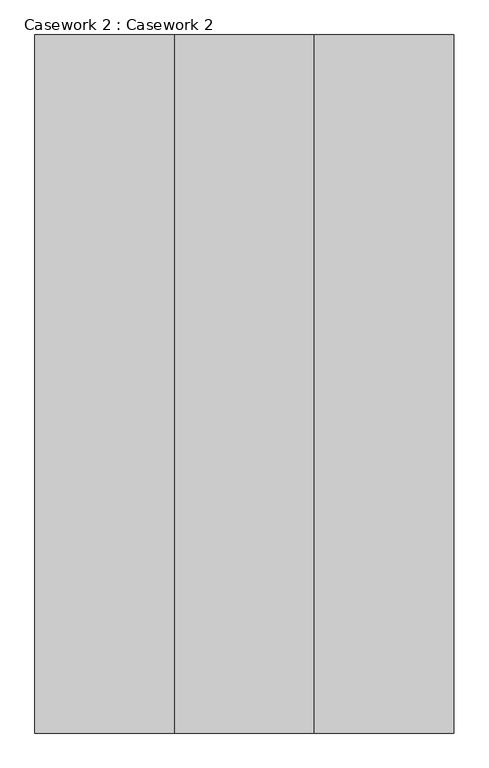
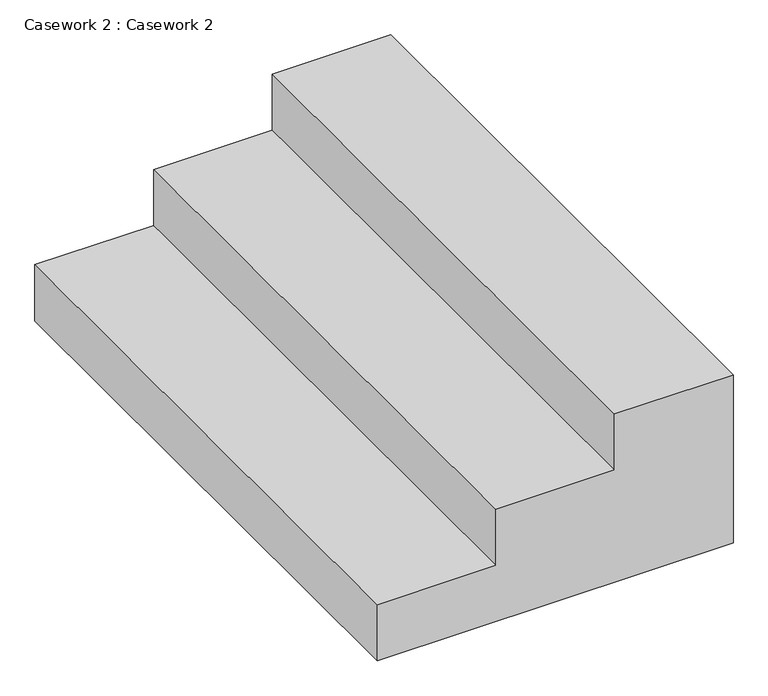
"""IFC4 building model written with IfcOpenShell, lengths in millimetres: furniture geometry, Casework 2 : Casework 2."""

from ifc_helpers import new_model, si_unit, frame, origin, place, context, project, spatial, polyline, outline, extrude, source, transform, mapped, element, save


def casework_2_casework_2_cc4890fd(model_context):
    return source(origin(), model_context, "Body", "SweptSolid", [
        extrude(outline(polyline([(1219.2, -5442.2469122), (1066.8, -5442.2469122), (1066.8, -5747.0469122), (914.4, -5747.0469122), (914.4, -6051.8469122), (762.0, -6051.8469122), (762.0, -5137.4469122), (1219.2, -5137.4469122), (1219.2, -5442.2469122)])), frame((0.0, 10596.9168074, 0.0), z_axis=(0.0, 1.0, 0.0), x_axis=(0.0, 0.0, 1.0)), (0.0, 0.0, 1.0), 1523.8525821),
    ])


if __name__ == "__main__":
    model = new_model("IFC4")
    model_context = context("Model", 3, world=origin())
    ifc_project = project(units=[si_unit("LENGTHUNIT", "METRE", prefix="MILLI")], contexts=[model_context])
    site = spatial("IfcSite", under=ifc_project)
    building = spatial("IfcBuilding", under=site)
    placement = place(None, origin())
    casework_2_casework_2_shape = casework_2_casework_2_cc4890fd(model_context)
    element("IfcFurniture", 1, ObjectType="Casework 2 : Casework 2", at=placement, inside=building, context=model_context, shape_type="MappedRepresentation", body=[
        mapped(casework_2_casework_2_shape, transform((0.0, 0.0, 0.0), x_axis=(1.0, 0.0, 0.0), y_axis=(0.0, 1.0, 0.0), z_axis=(0.0, 0.0, 1.0))),
    ])
    save(model, "model.ifc")
